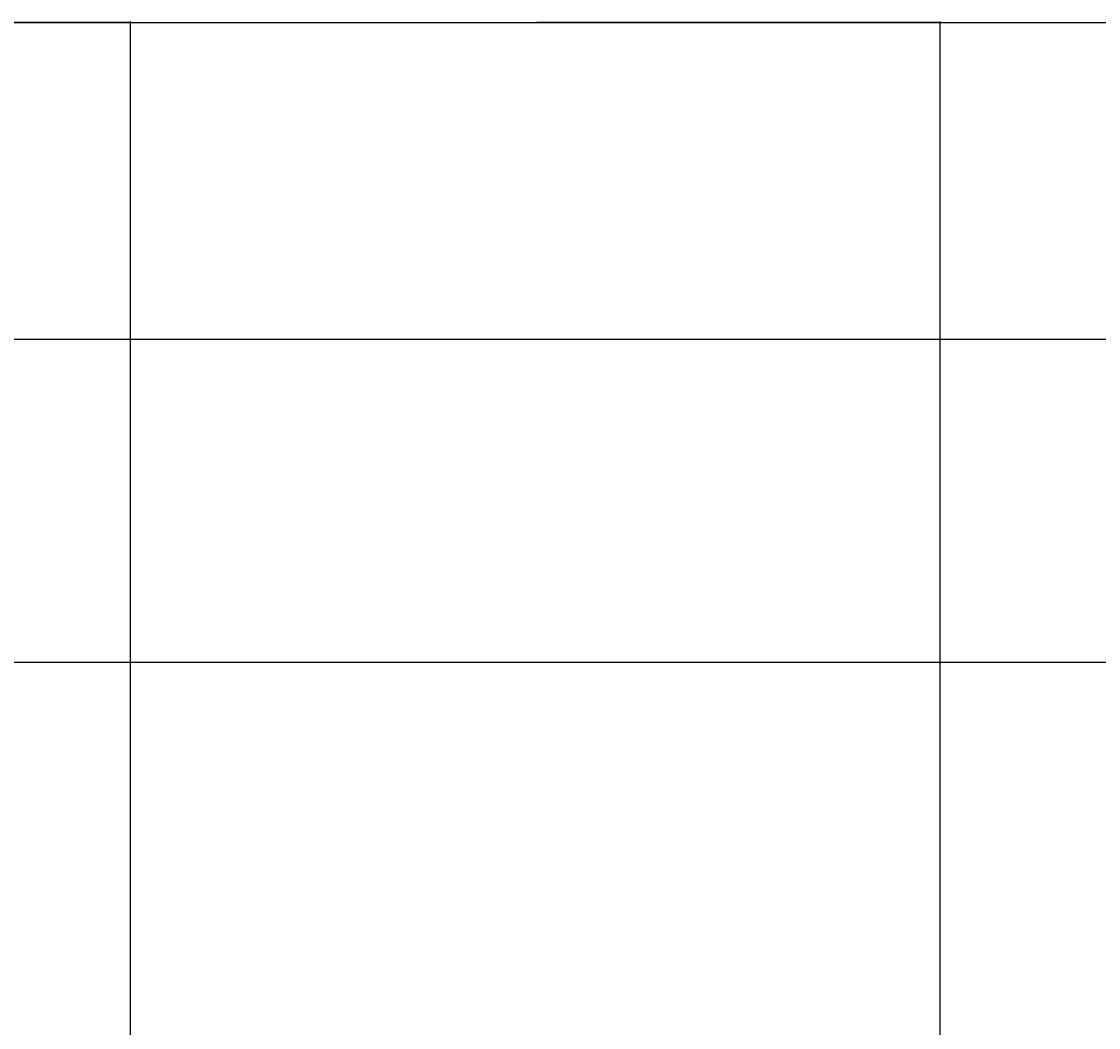
# Model space of a CAD drawing. Units: inches. Extents: x 1693 to 2974, y 2201 to 2965.
# Tile 14 of 24: x 1976 to 2175, y 2779 to 2965. Entities that reach past the tile are written whole.
import ezdxf

# ---------------------------------------------------------------- set-up
doc = ezdxf.new("R2010")
doc.units = ezdxf.units.IN
doc.header["$LTSCALE"] = 2
doc.header["$MEASUREMENT"] = 0
doc.layers.add('A-ANNO-DIMS', color=2, linetype='Continuous', lineweight=18)
doc.styles.get("Standard").update_dxf_attribs({"font": 'arial.ttf'})
doc.dimstyles.get("Standard").update_dxf_attribs({"dimtxt": 0.18, "dimasz": 0.18, "dimexe": 0.18, "dimexo": 0.0625, "dimgap": 0.09, "dimtad": 0, "dimtih": 1, "dimtoh": 1, "dimdec": 1, "dimzin": 0, "dimdsep": 46, "dimlunit": 3, "dimtxsty": 'Standard', "dimcen": 0.09, "dimadec": 0, "dimazin": 0, "dimtfac": 1, "dimtdec": 1, "dimtofl": 0, "dimtmove": 0, "dimatfit": 3, "dimfxl": 1, "dimtolj": 1, "dimtzin": 0, "dimarcsym": 0})

# ---------------------------------------------------------------- blocks, each defined once
blk = doc.blocks.new('*D81')
at = {"layer": 'A-ANNO-DIMS', "color": 0, "lineweight": -2, "ltscale": 2, "transparency": 16777216}
for p, q in [((1752.34, 2553.91), (1752.34, 2964.96)), ((1752.52, 2964.78), (2332.94, 2964.78)), ((2914.06, 2964.78), (2333.64, 2964.78)), ((2914.24, 2754.97), (2914.24, 2964.96))]:
    blk.add_line(p, q, dxfattribs=at)
at = {"layer": 'A-ANNO-DIMS', "color": 0, "ltscale": 2, "transparency": 16777216}
for points in [[(1752.52, 2964.81), (1752.52, 2964.75), (1752.34, 2964.78)], [(2914.06, 2964.81), (2914.06, 2964.75), (2914.24, 2964.78)]]:
    blk.add_solid(points, dxfattribs=at)
at = {"layer": 'Defpoints', "color": 0, "ltscale": 2, "transparency": 16777216}
for p in [(2914.24, 2964.78), (2914.24, 2754.9), (1752.34, 2553.84)]:
    blk.add_point(p, dxfattribs=at)
at = {"layer": 'A-ANNO-DIMS', "color": 0, "ltscale": 2, "transparency": 16777216, "insert": (2333.29, 2964.78), "char_height": 0.18, "attachment_point": 5}
blk.add_mtext('\\A1;1162', dxfattribs=at)
blk = doc.blocks.new('*D82')
at = {"layer": 'A-ANNO-DIMS', "color": 0, "lineweight": -2, "ltscale": 2, "transparency": 16777216}
for p, q in [((2615.67, 2906.08), (1693.46, 2906.08)), ((1693.64, 2905.9), (1693.64, 2582.94)), ((1693.64, 2259.62), (1693.64, 2582.58)), ((2096.17, 2259.44), (1693.46, 2259.44))]:
    blk.add_line(p, q, dxfattribs=at)
at = {"layer": 'A-ANNO-DIMS', "color": 0, "ltscale": 2, "transparency": 16777216}
for points in [[(1693.61, 2905.9), (1693.67, 2905.9), (1693.64, 2906.08)], [(1693.61, 2259.62), (1693.67, 2259.62), (1693.64, 2259.44)]]:
    blk.add_solid(points, dxfattribs=at)
at = {"layer": 'Defpoints', "color": 0, "ltscale": 2, "transparency": 16777216}
for p in [(1693.64, 2906.08), (2615.74, 2906.08), (2096.24, 2259.44)]:
    blk.add_point(p, dxfattribs=at)
at = {"layer": 'A-ANNO-DIMS', "color": 0, "ltscale": 2, "transparency": 16777216, "insert": (1693.64, 2582.76), "char_height": 0.18, "attachment_point": 5}
blk.add_mtext('\\A1;646.6', dxfattribs=at)
blk = doc.blocks.new('*D91')
at = {"layer": 'A-ANNO-DIMS', "color": 0, "lineweight": -2, "ltscale": 2, "transparency": 16777216}
for p, q in [((2615.67, 2906.08), (1693.46, 2906.08)), ((1693.64, 2905.9), (1693.64, 2876.35)), ((1693.64, 2846.43), (1693.64, 2875.98)), ((2479.17, 2846.25), (1693.46, 2846.25))]:
    blk.add_line(p, q, dxfattribs=at)
at = {"layer": 'A-ANNO-DIMS', "color": 0, "ltscale": 2, "transparency": 16777216}
for points in [[(1693.61, 2905.9), (1693.67, 2905.9), (1693.64, 2906.08)], [(1693.61, 2846.43), (1693.67, 2846.43), (1693.64, 2846.25)]]:
    blk.add_solid(points, dxfattribs=at)
at = {"layer": 'Defpoints', "color": 0, "ltscale": 2, "transparency": 16777216}
for p in [(2615.74, 2906.08), (1693.64, 2846.25), (2479.24, 2846.25)]:
    blk.add_point(p, dxfattribs=at)
at = {"layer": 'A-ANNO-DIMS', "color": 0, "ltscale": 2, "transparency": 16777216, "insert": (1693.64, 2876.17), "char_height": 0.18, "attachment_point": 5}
blk.add_mtext('\\A1;59.82', dxfattribs=at)
blk = doc.blocks.new('*D103')
at = {"layer": 'A-ANNO-DIMS', "color": 0, "lineweight": -2, "ltscale": 2, "transparency": 16777216}
for p, q in [((1923.74, 2737.28), (1923.74, 2964.96)), ((1923.92, 2964.78), (1959.52, 2964.78)), ((1995.56, 2964.78), (1959.95, 2964.78)), ((1995.74, 2737.28), (1995.74, 2964.96))]:
    blk.add_line(p, q, dxfattribs=at)
at = {"layer": 'A-ANNO-DIMS', "color": 0, "ltscale": 2, "transparency": 16777216}
for points in [[(1923.92, 2964.81), (1923.92, 2964.75), (1923.74, 2964.78)], [(1995.56, 2964.81), (1995.56, 2964.75), (1995.74, 2964.78)]]:
    blk.add_solid(points, dxfattribs=at)
at = {"layer": 'Defpoints', "color": 0, "ltscale": 2, "transparency": 16777216}
for p in [(1995.74, 2964.78), (1923.74, 2737.22), (1995.74, 2737.22)]:
    blk.add_point(p, dxfattribs=at)
at = {"layer": 'A-ANNO-DIMS', "color": 0, "ltscale": 2, "transparency": 16777216, "insert": (1959.74, 2964.78), "char_height": 0.18, "attachment_point": 5}
blk.add_mtext('\\A1;72', dxfattribs=at)
blk = doc.blocks.new('*D104')
at = {"layer": 'A-ANNO-DIMS', "color": 0, "lineweight": -2, "ltscale": 2, "transparency": 16777216}
for p, q in [((1995.74, 2747.41), (1995.74, 2964.96)), ((1995.92, 2964.78), (2070.46, 2964.78)), ((2145.56, 2964.78), (2071.02, 2964.78)), ((2145.74, 2774.6), (2145.74, 2964.96))]:
    blk.add_line(p, q, dxfattribs=at)
at = {"layer": 'A-ANNO-DIMS', "color": 0, "ltscale": 2, "transparency": 16777216}
for points in [[(1995.92, 2964.81), (1995.92, 2964.75), (1995.74, 2964.78)], [(2145.56, 2964.81), (2145.56, 2964.75), (2145.74, 2964.78)]]:
    blk.add_solid(points, dxfattribs=at)
at = {"layer": 'Defpoints', "color": 0, "ltscale": 2, "transparency": 16777216}
for p in [(2145.74, 2964.78), (2145.74, 2774.54), (1995.74, 2747.34)]:
    blk.add_point(p, dxfattribs=at)
at = {"layer": 'A-ANNO-DIMS', "color": 0, "ltscale": 2, "transparency": 16777216, "insert": (2070.74, 2964.78), "char_height": 0.18, "attachment_point": 5}
blk.add_mtext('\\A1;150', dxfattribs=at)

msp = doc.modelspace()

# ---------------------------------------------------------------- dimensions: what is measured, and where the dimension line sits
at = {"layer": 'A-ANNO-DIMS', "ltscale": 2}
for base, p1, p2, picture, middle in [((2914.2363, 2964.7761), (1752.3363, 2553.8449), (2914.2363, 2754.903), '*D81', (2333.2863, 2964.7761)), ((1995.7363, 2964.7761), (1923.7363, 2737.2161), (1995.7363, 2737.2161), '*D103', (1959.7363, 2964.7761)), ((2145.7363, 2964.7761), (1995.7363, 2747.3449), (2145.7363, 2774.5394), '*D104', (2070.7363, 2964.7761))]:
    dim = msp.add_linear_dim(base=base, p1=p1, p2=p2, dimstyle='Standard', override={"dimdec": 0, "dimlfac": 1, "dimrnd": 0, "dimzin": 0, "dimdsep": 46, "dimlunit": 2}, dxfattribs=at)
    dim.commit()
    dim.dimension.update_dxf_attribs({"geometry": picture, "text_midpoint": middle})
for base, p1, p2, override, picture, middle in [((1693.6363, 2906.0761), (2096.2363, 2259.4449), (2615.7363, 2906.0761), {"dimdec": 1, "dimlfac": 1, "dimrnd": 0, "dimzin": 0, "dimdsep": 46, "dimlunit": 2}, '*D82', (1693.6363, 2582.7605)), ((1693.6363, 2846.2547), (2615.7363, 2906.0761), (2479.2363, 2846.2547), {"dimdec": 2, "dimlfac": 1, "dimrnd": 0, "dimzin": 0, "dimdsep": 46, "dimlunit": 2}, '*D91', (1693.6363, 2876.1654))]:
    dim = msp.add_linear_dim(base=base, p1=p1, p2=p2, angle=90, dimstyle='Standard', override=override, dxfattribs=at)
    dim.commit()
    dim.dimension.update_dxf_attribs({"geometry": picture, "text_midpoint": middle})

doc.saveas('drawing.dxf')
